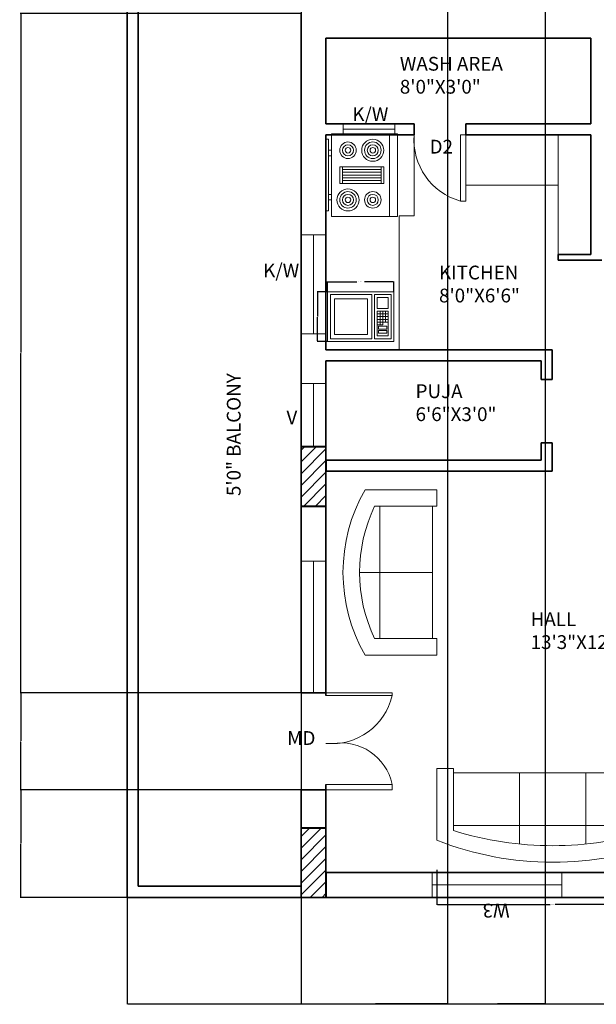
# Model space of a CAD drawing. Units: inches. Extents: x -86 to 2463, y -1058 to 68.
# Tile 1 of 17: x -86 to 123, y -740 to -383. Entities that reach past the tile are written whole.
import ezdxf

# ---------------------------------------------------------------- set-up
doc = ezdxf.new("R2010")
doc.units = ezdxf.units.IN
doc.header["$MEASUREMENT"] = 0
for name, color, linetype, lineweight in [('A-ANNO-DIMS', 2, 'Continuous', 18), ('A-ANNO-TEXT', 7, 'Continuous', 18), ('A-AREA-IDEN', 7, 'Continuous', 18), ('A-COLS', 7, 'Continuous', 40), ('A-COLS-PATT', 252, 'Continuous', 13), ('A-DOOR', 3, 'Continuous', 18), ('A-EQPM', 9, 'Continuous', 18), ('A-FLOR-CASE', 8, 'Continuous', 18), ('A-FURN', 8, 'Continuous', 18), ('A-GLAZ', 4, 'Continuous', 18), ('A-WALL', 7, 'Continuous', 35)]:
    doc.layers.add(name, color=color, linetype=linetype, lineweight=lineweight)
doc.styles.get("Standard").update_dxf_attribs({"font": 'arial.ttf'})
doc.dimstyles.get("Standard").update_dxf_attribs({"dimtxt": 0.18, "dimasz": 0.18, "dimexe": 0.18, "dimexo": 0.0625, "dimgap": 0.09, "dimtad": 0, "dimtih": 1, "dimtoh": 1, "dimdec": 4, "dimzin": 0, "dimdsep": 46, "dimtxsty": 'Standard', "dimcen": 0.09, "dimadec": 0, "dimazin": 0, "dimtfac": 1, "dimtdec": 4, "dimtofl": 0, "dimtmove": 0, "dimatfit": 3, "dimfxl": 1, "dimtolj": 1, "dimtzin": 0, "dimarcsym": 0})
pattern_1 = [(45, (-1015.1314, -586.0864), (-2.1213203, 2.1213203), [])]

# ---------------------------------------------------------------- blocks, each defined once
blk = doc.blocks.new('Sofa - Roundback 7 ft.')
for p, q in [((-12.00002, -32.4421), (-12.00003, -6.5971)), ((11.99997, -32.4421), (11.99998, -6.5971)), ((-36.000027, -34), (-36.000027, -11.4696)), ((-35.999844, -13.3819), (35.9998, -13.3819)), ((35.99998, -34), (35.99998, -11.4696)), ((-36.000027, -32.4421), (35.99998, -32.4421))]:
    blk.add_line(p, q)
for points in [[(-36.000027, -34), (-42.000027, -34), (-42.000027, -8)], [(41.99998, -8), (41.99998, -34), (35.99998, -34)]]:
    blk.add_lwpolyline(points)
for centre, radius, start, end in [((0, -114.25), 114.25, 68.43141, 111.5686), ((-0.00001, -127.1968), 121.1968, 72.72033, 107.2797)]:
    blk.add_arc(centre, radius, start, end)
blk = doc.blocks.new('Sofa - Roundback Loveseat 5 ft.')
for p, q in [((0, -32.44198), (0, -5.99998)), ((-24, -33.99998), (-24, -11.46958)), ((-23.9998, -13.38178), (23.99986, -13.38178)), ((24.00004, -33.99998), (24.00004, -11.46958)), ((-24, -32.44198), (24.00004, -32.44198))]:
    blk.add_line(p, q)
for points in [[(-24, -33.99998), (-30, -33.99998), (-30, -7.99998)], [(30.00004, -7.99998), (30.00004, -33.99998), (24.00004, -33.99998)]]:
    blk.add_lwpolyline(points)
for centre, radius, start, end in [((0, -60.24998), 60.24998, 60.13715, 119.8628), ((0, -61.38438), 55.38444, 64.32083, 115.6792)]:
    blk.add_arc(centre, radius, start, end)
blk = doc.blocks.new('Range-Oven - 30 in top')
for p, q in [((0, -3), (30, -3)), ((12, -6), (18, -6)), ((13, -20), (13, -6)), ((14, -6), (14, -20)), ((15, -20), (15, -6)), ((16, -6), (16, -20)), ((17, -20), (17, -6)), ((18, -20), (12, -20)), ((6, -24), (6, -25)), ((8, -25), (8, -24)), ((22, -25), (22, -24)), ((24, -24), (24, -25))]:
    blk.add_line(p, q)
for points in [[(0, -24), (0, 0), (30, 0), (30, -24)], [(12, -21), (12, -5), (18, -5), (18, -21)], [(2, -26), (2, -25), (28, -25), (28, -26)]]:
    blk.add_lwpolyline(points, close=True)
for centre, radius in [((6, -9), 4), ((6, -9), 3), ((6, -9), 2), ((24, -9), 3), ((24, -9), 2), ((6, -9), 1), ((24, -9), 1), ((24, -18), 4), ((6, -18), 3), ((6, -18), 2), ((6, -18), 1), ((24, -18), 3), ((24, -18), 2), ((24, -18), 1)]:
    blk.add_circle(centre, radius)
blk = doc.blocks.new('Microwave')
for p, q in [((19, 7), (19, 11)), ((20, 11), (20, 7)), ((21, 7), (21, 11)), ((18, 10), (22, 10)), ((22, 9), (18, 9)), ((18, 8), (22, 8)), ((22, 7), (18, 7)), ((20, 6), (18, 6)), ((19, 6), (19, 7)), ((20, 7), (20, 6))]:
    blk.add_line(p, q)
for points in [[(0, 0), (0, 18), (24, 18), (24, 0)], [(1, 1), (1, 17), (16, 17), (16, 1)], [(2.5, 2.5), (2.5, 15.5), (14.5, 15.5), (14.5, 2.5)], [(17, 1), (17, 17), (23, 17), (23, 1)], [(18, 12), (18, 16), (22, 16), (22, 12)], [(18, 2), (18, 11), (22, 11), (22, 2)], [(18.5, 4.5), (18.5, 5.5), (21.5, 5.5), (21.5, 4.5)], [(18.5, 3), (18.5, 4), (21.5, 4), (21.5, 3)]]:
    blk.add_lwpolyline(points, close=True)
blk = doc.blocks.new('*D14')
at = {"layer": 'A-ANNO-DIMS', "color": 0, "lineweight": -2, "transparency": 16777216}
for p, q in [((25.37, -481.97), (25.37, -478.25)), ((49.37, -481.97), (49.37, -478.25)), ((25.55, -478.43), (36.02, -478.43)), ((49.19, -478.43), (38.72, -478.43))]:
    blk.add_line(p, q, dxfattribs=at)
at = {"layer": 'A-ANNO-DIMS', "color": 0, "transparency": 16777216}
for points in [[(25.55, -478.4), (25.55, -478.46), (25.37, -478.43)], [(49.19, -478.4), (49.19, -478.46), (49.37, -478.43)]]:
    blk.add_solid(points, dxfattribs=at)
at = {"layer": 'Defpoints', "color": 0, "transparency": 16777216}
for p in [(49.37, -478.43), (25.37, -482.03), (49.37, -482.03)]:
    blk.add_point(p, dxfattribs=at)
at = {"layer": 'A-ANNO-DIMS', "color": 0, "transparency": 16777216, "insert": (37.37, -478.43), "char_height": 0.18, "attachment_point": 5}
blk.add_mtext('\\A1;MICROWAVE 24 TYP.', dxfattribs=at)
blk = doc.blocks.new('*D15')
at = {"layer": 'A-ANNO-DIMS', "color": 0, "lineweight": -2, "transparency": 16777216}
for p, q in [((25.31, -482.03), (21.59, -482.03)), ((21.77, -482.21), (21.77, -490.85)), ((21.77, -499.85), (21.77, -491.21)), ((25.31, -500.03), (21.59, -500.03))]:
    blk.add_line(p, q, dxfattribs=at)
at = {"layer": 'A-ANNO-DIMS', "color": 0, "transparency": 16777216}
for points in [[(21.74, -482.21), (21.8, -482.21), (21.77, -482.03)], [(21.74, -499.85), (21.8, -499.85), (21.77, -500.03)]]:
    blk.add_solid(points, dxfattribs=at)
at = {"layer": 'Defpoints', "color": 0, "transparency": 16777216}
for p in [(21.77, -482.03), (25.37, -482.03), (25.37, -500.03)]:
    blk.add_point(p, dxfattribs=at)
at = {"layer": 'A-ANNO-DIMS', "color": 0, "transparency": 16777216, "insert": (21.77, -491.03), "char_height": 0.18, "attachment_point": 5}
blk.add_mtext('\\A1;18 TYP.', dxfattribs=at)
blk = doc.blocks.new('*D26')
at = {"layer": 'A-ANNO-DIMS', "color": 0, "lineweight": -2, "transparency": 16777216}
for p, q in [((64.97, -691.61), (64.97, -704.32)), ((148.97, -691.61), (148.97, -704.32)), ((65.15, -704.14), (106.07, -704.14)), ((148.79, -704.14), (107.88, -704.14))]:
    blk.add_line(p, q, dxfattribs=at)
at = {"layer": 'A-ANNO-DIMS', "color": 0, "transparency": 16777216}
for points in [[(65.15, -704.11), (65.15, -704.17), (64.97, -704.14)], [(148.79, -704.11), (148.79, -704.17), (148.97, -704.14)]]:
    blk.add_solid(points, dxfattribs=at)
at = {"layer": 'Defpoints', "color": 0, "transparency": 16777216}
for p in [(64.97, -691.54), (148.97, -691.54), (64.97, -704.14)]:
    blk.add_point(p, dxfattribs=at)
at = {"layer": 'A-ANNO-DIMS', "color": 0, "transparency": 16777216, "insert": (106.97, -704.14), "char_height": 0.18, "attachment_point": 5}
blk.add_mtext('\\A1;SOFA 84 TYP.', dxfattribs=at)
blk = doc.blocks.new('*D30')
at = {"layer": 'A-ANNO-DIMS', "color": 0, "lineweight": -2, "transparency": 16777216}
for p, q in [((-47.24, -701.67), (-47.24, -740.38)), ((386.76, -701.67), (386.76, -740.38)), ((-47.06, -740.2), (169.47, -740.2)), ((386.58, -740.2), (170.05, -740.2))]:
    blk.add_line(p, q, dxfattribs=at)
at = {"layer": 'A-ANNO-DIMS', "color": 0, "transparency": 16777216}
for points in [[(-47.06, -740.17), (-47.06, -740.23), (-47.24, -740.2)], [(386.58, -740.17), (386.58, -740.23), (386.76, -740.2)]]:
    blk.add_solid(points, dxfattribs=at)
at = {"layer": 'Defpoints', "color": 0, "transparency": 16777216}
for p in [(-47.24, -701.6), (386.76, -701.6), (386.76, -740.2)]:
    blk.add_point(p, dxfattribs=at)
at = {"layer": 'A-ANNO-DIMS', "color": 0, "transparency": 16777216, "insert": (169.76, -740.2), "char_height": 0.18, "attachment_point": 5}
blk.add_mtext('\\A1;434', dxfattribs=at)
blk = doc.blocks.new('*D33')
at = {"layer": 'A-ANNO-DIMS', "color": 0, "lineweight": -2, "transparency": 16777216}
for p, q in [((15.7, -381.1), (-86.02, -381.1)), ((-85.84, -381.28), (-85.84, -504.09)), ((-85.84, -627.25), (-85.84, -504.45)), ((15.7, -627.43), (-86.02, -627.43))]:
    blk.add_line(p, q, dxfattribs=at)
at = {"layer": 'A-ANNO-DIMS', "color": 0, "transparency": 16777216}
for points in [[(-85.87, -381.28), (-85.81, -381.28), (-85.84, -381.1)], [(-85.87, -627.25), (-85.81, -627.25), (-85.84, -627.43)]]:
    blk.add_solid(points, dxfattribs=at)
at = {"layer": 'Defpoints', "color": 0, "transparency": 16777216}
for p in [(-85.84, -381.1), (15.76, -381.1), (15.76, -627.43)]:
    blk.add_point(p, dxfattribs=at)
at = {"layer": 'A-ANNO-DIMS', "color": 0, "transparency": 16777216, "insert": (-85.84, -504.27), "char_height": 0.18, "attachment_point": 5}
blk.add_mtext('\\A1;246.33', dxfattribs=at)
blk = doc.blocks.new('*D39')
at = {"layer": 'A-ANNO-DIMS', "color": 0, "lineweight": -2, "transparency": 16777216}
for p, q in [((15.7, -662.64), (-86.02, -662.64)), ((-85.84, -662.82), (-85.84, -681.94)), ((-85.84, -701.42), (-85.84, -682.3)), ((15.7, -701.6), (-86.02, -701.6))]:
    blk.add_line(p, q, dxfattribs=at)
at = {"layer": 'A-ANNO-DIMS', "color": 0, "transparency": 16777216}
for points in [[(-85.87, -662.82), (-85.81, -662.82), (-85.84, -662.64)], [(-85.87, -701.42), (-85.81, -701.42), (-85.84, -701.6)]]:
    blk.add_solid(points, dxfattribs=at)
at = {"layer": 'Defpoints', "color": 0, "transparency": 16777216}
for p in [(-85.84, -662.64), (15.76, -662.64), (15.76, -701.6)]:
    blk.add_point(p, dxfattribs=at)
at = {"layer": 'A-ANNO-DIMS', "color": 0, "transparency": 16777216, "insert": (-85.84, -682.12), "char_height": 0.18, "attachment_point": 5}
blk.add_mtext('\\A1;38.96', dxfattribs=at)
blk = doc.blocks.new('*D40')
at = {"layer": 'A-ANNO-DIMS', "color": 0, "lineweight": -2, "transparency": 16777216}
for p, q in [((15.7, -627.43), (-86.02, -627.43)), ((-85.84, -627.61), (-85.84, -644.86)), ((-85.84, -662.46), (-85.84, -645.22)), ((15.7, -662.64), (-86.02, -662.64))]:
    blk.add_line(p, q, dxfattribs=at)
at = {"layer": 'A-ANNO-DIMS', "color": 0, "transparency": 16777216}
for points in [[(-85.87, -627.61), (-85.81, -627.61), (-85.84, -627.43)], [(-85.87, -662.46), (-85.81, -662.46), (-85.84, -662.64)]]:
    blk.add_solid(points, dxfattribs=at)
at = {"layer": 'Defpoints', "color": 0, "transparency": 16777216}
for p in [(-85.84, -627.43), (15.76, -627.43), (15.76, -662.64)]:
    blk.add_point(p, dxfattribs=at)
at = {"layer": 'A-ANNO-DIMS', "color": 0, "transparency": 16777216, "insert": (-85.84, -645.04), "char_height": 0.18, "attachment_point": 5}
blk.add_mtext('\\A1;35.21', dxfattribs=at)
blk = doc.blocks.new('*D41')
at = {"layer": 'A-ANNO-DIMS', "color": 0, "lineweight": -2, "transparency": 16777216}
for p, q in [((15.76, -303.17), (15.76, -740.38)), ((68.89, -303.17), (68.89, -740.38)), ((15.94, -740.2), (41.93, -740.2)), ((68.71, -740.2), (42.72, -740.2))]:
    blk.add_line(p, q, dxfattribs=at)
at = {"layer": 'A-ANNO-DIMS', "color": 0, "transparency": 16777216}
for points in [[(15.94, -740.17), (15.94, -740.23), (15.76, -740.2)], [(68.71, -740.17), (68.71, -740.23), (68.89, -740.2)]]:
    blk.add_solid(points, dxfattribs=at)
at = {"layer": 'Defpoints', "color": 0, "transparency": 16777216}
for p in [(15.76, -303.1), (68.89, -303.1), (68.89, -740.2)]:
    blk.add_point(p, dxfattribs=at)
at = {"layer": 'A-ANNO-DIMS', "color": 0, "transparency": 16777216, "insert": (42.33, -740.2), "char_height": 0.18, "attachment_point": 5}
blk.add_mtext('\\A1;53.13', dxfattribs=at)
blk = doc.blocks.new('*D42')
at = {"layer": 'A-ANNO-DIMS', "color": 0, "lineweight": -2, "transparency": 16777216}
for p, q in [((68.89, -303.17), (68.89, -740.38)), ((104.26, -303.17), (104.26, -740.38)), ((69.07, -740.2), (86.18, -740.2)), ((104.08, -740.2), (86.97, -740.2))]:
    blk.add_line(p, q, dxfattribs=at)
at = {"layer": 'A-ANNO-DIMS', "color": 0, "transparency": 16777216}
for points in [[(69.07, -740.17), (69.07, -740.23), (68.89, -740.2)], [(104.08, -740.17), (104.08, -740.23), (104.26, -740.2)]]:
    blk.add_solid(points, dxfattribs=at)
at = {"layer": 'Defpoints', "color": 0, "transparency": 16777216}
for p in [(68.89, -303.1), (104.26, -303.1), (104.26, -740.2)]:
    blk.add_point(p, dxfattribs=at)
at = {"layer": 'A-ANNO-DIMS', "color": 0, "transparency": 16777216, "insert": (86.58, -740.2), "char_height": 0.18, "attachment_point": 5}
blk.add_mtext('\\A1;35.37', dxfattribs=at)

msp = doc.modelspace()

# ---------------------------------------------------------------- hatches: boundary and pattern name
at = {"layer": 'A-COLS-PATT'}
h = msp.add_hatch(dxfattribs=at)
h.set_pattern_fill('ANSI31', color=256, scale=24)
h.set_pattern_definition(pattern_1)
h.paths.add_polyline_path([(386.761, -543.104), (377.846, -543.104), (377.846, -547.104), (377.846, -559.337), (386.761, -559.337)])
h.paths.add_polyline_path([(24.761, -547.104), (24.761, -543.104), (24.761, -538.166), (15.761, -538.166), (15.761, -559.72), (24.761, -559.72)])
h = msp.add_hatch(dxfattribs=at)
h.set_pattern_fill('ANSI31', color=256, scale=24)
h.set_pattern_definition(pattern_1)
h.paths.add_polyline_path([(24.761, -676.336), (15.761, -676.336), (15.761, -701.604), (24.761, -701.604), (24.761, -692.604)])
h.paths.add_polyline_path([(198.701, -692.604), (187.846, -692.604), (183.846, -692.604), (183.846, -701.604), (198.701, -701.604)])
h.paths.add_polyline_path([(386.761, -684.448), (377.846, -684.448), (377.846, -692.604), (377.846, -701.604), (386.761, -701.604)])

# ---------------------------------------------------------------- linework, layer by layer
at = {"layer": 'A-COLS'}
for p, q in [((15.761, -538.166), (24.761, -538.166)), ((24.761, -543.104), (24.761, -547.104)), ((15.761, -559.72), (24.761, -559.72)), ((15.761, -676.336), (24.761, -676.336)), ((24.761, -692.604), (24.761, -701.604))]:
    msp.add_line(p, q, dxfattribs=at)
at = {"layer": 'A-DOOR'}
for p, q in [((73.507, -449.104), (73.507, -425.104)), ((73.507, -425.104), (75.507, -425.104)), ((75.507, -425.104), (75.507, -449.104)), ((74.507, -449.104), (73.507, -449.104)), ((75.507, -449.104), (74.507, -449.104)), ((24.761, -627.432), (48.761, -627.432)), ((48.761, -627.432), (48.761, -628.432)), ((48.761, -628.432), (24.761, -628.432)), ((48.761, -660.642), (24.761, -660.642)), ((24.761, -662.642), (48.761, -662.642)), ((48.761, -662.642), (48.761, -660.642))]:
    msp.add_line(p, q, dxfattribs=at)
for centre, radius, start, end in [((79.699, -426.923), 23.029, 175.46946, 254.40337), ((26.935, -623.493), 22.377, 264.4229, 347.24812), ((30.231, -664.51), 18.929, 11.79317, 100.027)]:
    msp.add_arc(centre, radius, start, end, dxfattribs=at)
at = {"layer": 'A-FLOR-CASE'}
for p, q in [((56.742, -423.104), (56.742, -454.477)), ((108.954, -468.471), (108.954, -425.104)), ((108.954, -443.352), (75.507, -443.352)), ((56.742, -454.477), (51.259, -454.477)), ((51.259, -454.477), (51.259, -503.104))]:
    msp.add_line(p, q, dxfattribs=at)
at = {"layer": 'A-GLAZ'}
for p, q in [((30.972, -421.104), (30.972, -425.104)), ((49.691, -421.104), (49.691, -425.104)), ((30.972, -423.104), (49.691, -423.104)), ((15.761, -461.34), (24.761, -461.34)), ((20.261, -461.34), (20.261, -497.319)), ((24.761, -497.319), (15.761, -497.319)), ((15.761, -515.289), (24.761, -515.289)), ((20.261, -515.289), (20.261, -538.166)), ((15.761, -579.712), (24.761, -579.712)), ((20.261, -579.712), (20.261, -627.432)), ((63.24, -692.604), (63.24, -701.604)), ((110.262, -692.604), (110.262, -701.604)), ((63.24, -697.104), (110.262, -697.104))]:
    msp.add_line(p, q, dxfattribs=at)
at = {"layer": 'A-WALL'}
for p, q in [((-47.239, -141.104), (-47.239, -701.604)), ((-43.239, -141.104), (-43.239, -697.604)), ((15.761, -381.104), (15.761, -627.432)), ((24.761, -390.104), (24.761, -421.104)), ((120.761, -390.104), (24.761, -390.104)), ((120.761, -390.104), (120.761, -421.104)), ((56.742, -421.104), (24.761, -421.104)), ((56.742, -421.104), (56.742, -425.104)), ((120.761, -421.104), (75.507, -421.104)), ((75.507, -421.104), (75.507, -425.104)), ((24.761, -425.104), (24.761, -503.104)), ((56.742, -425.104), (24.761, -425.104)), ((120.761, -425.104), (75.507, -425.104)), ((120.761, -425.104), (120.761, -468.471)), ((108.954, -470.557), (108.954, -468.471)), ((108.954, -468.471), (120.761, -468.471)), ((120.761, -470.557), (108.954, -470.557)), ((120.761, -470.557), (124.761, -470.557)), ((106.761, -503.104), (24.761, -503.104)), ((106.761, -507.104), (106.761, -503.104)), ((24.761, -507.104), (24.761, -543.104)), ((102.761, -507.104), (24.761, -507.104)), ((102.761, -507.104), (102.761, -513.79)), ((106.761, -507.104), (106.761, -513.79)), ((102.761, -513.79), (106.761, -513.79)), ((102.761, -536.808), (106.761, -536.808)), ((102.761, -536.808), (102.761, -543.104)), ((106.761, -536.808), (106.761, -547.104)), ((102.761, -543.104), (24.761, -543.104)), ((106.761, -547.104), (24.761, -547.104)), ((24.761, -547.104), (24.761, -628.432)), ((15.761, -627.432), (24.761, -627.432)), ((15.761, -662.642), (24.761, -662.642)), ((15.761, -662.642), (15.761, -701.604)), ((24.761, -660.642), (24.761, -692.604)), ((183.846, -692.604), (24.761, -692.604)), ((-43.239, -697.604), (15.761, -697.604)), ((-47.239, -701.604), (15.761, -701.604)), ((386.761, -701.604), (15.761, -701.604))]:
    msp.add_line(p, q, dxfattribs=at)

# ---------------------------------------------------------------- block references
at = {"layer": 'A-EQPM', "rotation": 270}
msp.add_blockref('Range-Oven - 30 in top', (50.761, -424.696), dxfattribs=at)
at = {"layer": 'A-EQPM'}
msp.add_blockref('Microwave', (25.369, -500.033), dxfattribs=at)
at = {"layer": 'A-FURN'}
for name, p, rotation in [('Sofa - Roundback Loveseat 5 ft.', (30.957, -583.776), 90), ('Sofa - Roundback 7 ft.', (106.975, -688.878), 180)]:
    msp.add_blockref(name, p, dxfattribs=dict(at, rotation=rotation))

# ---------------------------------------------------------------- texts
at = {"layer": 'A-ANNO-TEXT', "char_height": 5, "attachment_point": 1}
for s, width, insert in [('K/W', 16.67426, (34.332, -415.127)), ('D2', 6.14385, (62.349, -426.904)), ('K/W', 6.94235, (2.031, -471.789)), ('V', 10.41352, (10.459, -525.081)), ('MD', 7.82676, (10.745, -641.337))]:
    msp.add_mtext_dynamic_manual_height_columns(s, width=width, gutter_width=25, heights=[0], dxfattribs=dict(at, insert=insert))
at = {"layer": 'A-ANNO-TEXT', "insert": (91.347, -708.918), "char_height": 5, "attachment_point": 1, "rotation": 180}
msp.add_mtext_dynamic_manual_height_columns('W3', width=16.65046, gutter_width=25, heights=[0], dxfattribs=at)
at = {"layer": 'A-AREA-IDEN', "char_height": 5, "attachment_point": 1}
for s, width, insert in [('WASH AREA\\P8\'0"X3\'0"', 81.49318, (51.56, -396.835)), ('KITCHEN\\P8\'0"X6\'6"', 82.94225, (65.761, -472.537)), ('PUJA\\P6\'6"X3\'0"', 37.67583, (57.26, -515.573)), ('HALL\\P13\'3"X12\'1.5"', 75.18459, (98.956, -598.214))]:
    msp.add_mtext_dynamic_manual_height_columns(s, width=width, gutter_width=25, heights=[0], dxfattribs=dict(at, insert=insert))
at = {"layer": 'A-AREA-IDEN', "insert": (-11.148, -556.094), "char_height": 5, "attachment_point": 1, "rotation": 90}
msp.add_mtext_dynamic_manual_height_columns('5\'0" BALCONY', width=106.5034, gutter_width=25, heights=[0], dxfattribs=at)

# ---------------------------------------------------------------- dimensions: what is measured, and where the dimension line sits
at = {"layer": 'A-ANNO-DIMS'}
for base, p1, p2, override, picture, middle in [((68.889, -740.204), (15.761, -303.104), (68.889, -303.104), {"dimdec": 2, "dimlfac": 1, "dimrnd": 0, "dimzin": 0, "dimdsep": 46, "dimlunit": 2}, '*D41', (42.325, -740.204)), ((104.261, -740.204), (68.889, -303.104), (104.261, -303.104), {"dimdec": 2, "dimlfac": 1, "dimrnd": 0, "dimzin": 0, "dimdsep": 46, "dimlunit": 2}, '*D42', (86.575, -740.204)), ((386.761, -740.204), (-47.239, -701.604), (386.761, -701.604), {"dimdec": 0, "dimlfac": 1, "dimrnd": 0, "dimzin": 0, "dimdsep": 46, "dimlunit": 2}, '*D30', (169.761, -740.204))]:
    dim = msp.add_linear_dim(base=base, p1=p1, p2=p2, dimstyle='Standard', override=override, dxfattribs=at)
    dim.commit()
    dim.dimension.update_dxf_attribs({"geometry": picture, "text_midpoint": middle})
for base, p1, p2, picture, middle in [((-85.839, -381.104), (15.761, -627.432), (15.761, -381.104), '*D33', (-85.839, -504.268)), ((-85.839, -627.432), (15.761, -662.642), (15.761, -627.432), '*D40', (-85.839, -645.037)), ((-85.839, -662.642), (15.761, -701.604), (15.761, -662.642), '*D39', (-85.839, -682.123))]:
    dim = msp.add_linear_dim(base=base, p1=p1, p2=p2, angle=90, dimstyle='Standard', override={"dimdec": 2, "dimlfac": 1, "dimrnd": 0, "dimzin": 0, "dimdsep": 46, "dimlunit": 2}, dxfattribs=at)
    dim.commit()
    dim.dimension.update_dxf_attribs({"geometry": picture, "text_midpoint": middle})
dim = msp.add_linear_dim(base=(49.369, -478.433), p1=(25.369, -482.033), p2=(49.369, -482.033), text='MICROWAVE <> TYP.', dimstyle='Standard', override={"dimdec": 0, "dimlfac": 1, "dimrnd": 0, "dimzin": 0, "dimdsep": 46, "dimlunit": 2}, dxfattribs=at)
dim.commit()
dim.dimension.update_dxf_attribs({"geometry": '*D14', "text_midpoint": (37.369, -478.433)})
for base, p1, p2, angle, text, picture, middle in [((21.769, -482.033), (25.369, -500.033), (25.369, -482.033), 90, '<> TYP.', '*D15', (21.769, -491.033)), ((64.975, -704.145), (148.975, -691.545), (64.975, -691.545), 180, 'SOFA <> TYP.', '*D26', (106.975, -704.145))]:
    dim = msp.add_linear_dim(base=base, p1=p1, p2=p2, angle=angle, text=text, dimstyle='Standard', override={"dimdec": 0, "dimlfac": 1, "dimrnd": 0, "dimzin": 0, "dimdsep": 46, "dimlunit": 2}, dxfattribs=at)
    dim.commit()
    dim.dimension.update_dxf_attribs({"geometry": picture, "text_midpoint": middle})

doc.saveas('drawing.dxf')
